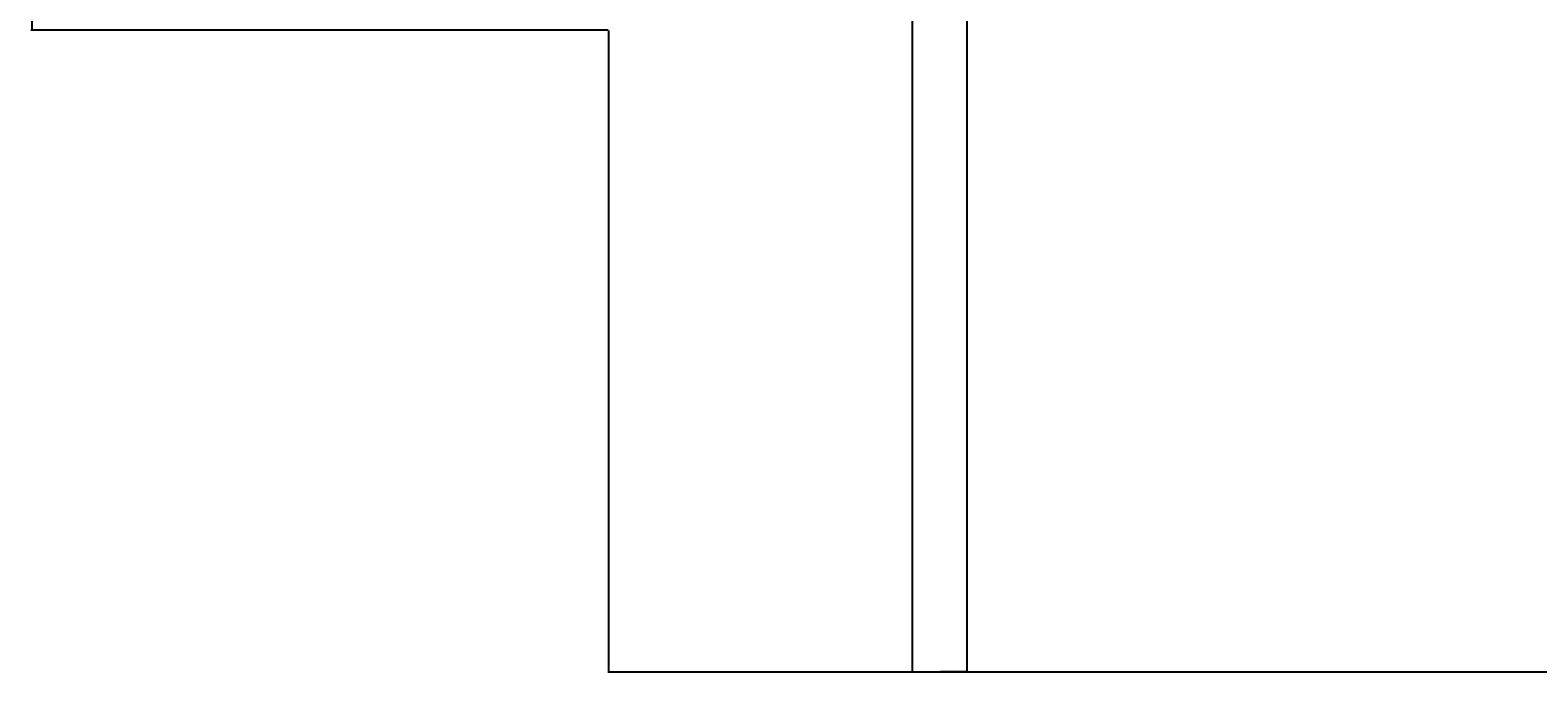
# Model space of a CAD drawing. Units: inches. Extents: x 5375 to 6084, y 16106 to 17259.
# Tile 1 of 32: x 5375 to 5624, y 16106 to 16212. Entities that reach past the tile are written whole.
import ezdxf

# ---------------------------------------------------------------- set-up
doc = ezdxf.new("R2010")
doc.units = ezdxf.units.IN
doc.layers.add('A-ANNO-DIMS', color=2, linetype='Continuous', lineweight=18)
doc.styles.get("Standard").update_dxf_attribs({"font": 'arial.ttf'})
doc.dimstyles.get("Standard").update_dxf_attribs({"dimtxt": 0.18, "dimasz": 0.18, "dimexe": 0.18, "dimexo": 0.0625, "dimgap": 0.09, "dimtad": 0, "dimtih": 1, "dimtoh": 1, "dimdec": 4, "dimzin": 0, "dimdsep": 46, "dimtxsty": 'Standard', "dimcen": 0.09, "dimadec": 0, "dimazin": 0, "dimtfac": 1, "dimtdec": 4, "dimtofl": 0, "dimtmove": 0, "dimatfit": 3, "dimfxl": 1, "dimtolj": 1, "dimtzin": 0, "dimarcsym": 0})

# ---------------------------------------------------------------- blocks, each defined once
blk = doc.blocks.new('*D30')
at = {"layer": 'A-ANNO-DIMS', "color": 0, "lineweight": -2, "transparency": 16777216}
for p, q in [((5470.62, 16212.32), (5470.62, 16106.48)), ((6031.62, 16212.32), (6031.62, 16106.48)), ((5470.8, 16106.66), (5750.85, 16106.66)), ((6031.44, 16106.66), (5751.39, 16106.66))]:
    blk.add_line(p, q, dxfattribs=at)
at = {"layer": 'A-ANNO-DIMS', "color": 0, "transparency": 16777216}
for points in [[(5470.8, 16106.69), (5470.8, 16106.63), (5470.62, 16106.66)], [(6031.44, 16106.69), (6031.44, 16106.63), (6031.62, 16106.66)]]:
    blk.add_solid(points, dxfattribs=at)
at = {"layer": 'Defpoints', "color": 0, "transparency": 16777216}
for p in [(5470.62, 16212.38), (6031.62, 16212.38), (6031.62, 16106.66)]:
    blk.add_point(p, dxfattribs=at)
at = {"layer": 'A-ANNO-DIMS', "color": 0, "transparency": 16777216, "insert": (5751.12, 16106.66), "char_height": 0.18, "attachment_point": 5}
blk.add_mtext('\\A1;561', dxfattribs=at)
blk = doc.blocks.new('*D33')
at = {"layer": 'A-ANNO-DIMS', "color": 0, "lineweight": -2, "transparency": 16777216}
for p, q in [((5470.56, 16360.58), (5375.56, 16360.58)), ((5375.74, 16360.4), (5375.74, 16286.66)), ((5375.74, 16212.56), (5375.74, 16286.3)), ((5470.56, 16212.38), (5375.56, 16212.38))]:
    blk.add_line(p, q, dxfattribs=at)
at = {"layer": 'A-ANNO-DIMS', "color": 0, "transparency": 16777216}
for points in [[(5375.71, 16360.4), (5375.77, 16360.4), (5375.74, 16360.58)], [(5375.71, 16212.56), (5375.77, 16212.56), (5375.74, 16212.38)]]:
    blk.add_solid(points, dxfattribs=at)
at = {"layer": 'Defpoints', "color": 0, "transparency": 16777216}
for p in [(5375.74, 16360.58), (5470.62, 16360.58), (5470.62, 16212.38)]:
    blk.add_point(p, dxfattribs=at)
at = {"layer": 'A-ANNO-DIMS', "color": 0, "transparency": 16777216, "insert": (5375.74, 16286.48), "char_height": 0.18, "attachment_point": 5}
blk.add_mtext('\\A1;148.2', dxfattribs=at)
blk = doc.blocks.new('*D40')
at = {"layer": 'A-ANNO-DIMS', "color": 0, "lineweight": -2, "transparency": 16777216}
for p, q in [((5529.62, 16876.52), (5529.62, 16106.48)), ((5520.62, 16867.52), (5520.62, 16106.48)), ((5520.8, 16106.66), (5524.97, 16106.66)), ((5529.44, 16106.66), (5525.27, 16106.66))]:
    blk.add_line(p, q, dxfattribs=at)
at = {"layer": 'A-ANNO-DIMS', "color": 0, "transparency": 16777216}
for points in [[(5520.8, 16106.69), (5520.8, 16106.63), (5520.62, 16106.66)], [(5529.44, 16106.69), (5529.44, 16106.63), (5529.62, 16106.66)]]:
    blk.add_solid(points, dxfattribs=at)
at = {"layer": 'Defpoints', "color": 0, "transparency": 16777216}
for p in [(5529.62, 16876.58), (5520.62, 16867.58), (5529.62, 16106.66)]:
    blk.add_point(p, dxfattribs=at)
at = {"layer": 'A-ANNO-DIMS', "color": 0, "transparency": 16777216, "insert": (5525.12, 16106.66), "char_height": 0.18, "attachment_point": 5}
blk.add_mtext('\\A1;9', dxfattribs=at)

msp = doc.modelspace()

# ---------------------------------------------------------------- dimensions: what is measured, and where the dimension line sits
at = {"layer": 'A-ANNO-DIMS'}
for base, p1, p2, picture, middle in [((5529.6199, 16106.6631), (5520.6199, 16867.5793), (5529.6199, 16876.5793), '*D40', (5525.1199, 16106.6631)), ((6031.6199, 16106.6631), (5470.6199, 16212.3785), (6031.6199, 16212.3785), '*D30', (5751.1199, 16106.6631))]:
    dim = msp.add_linear_dim(base=base, p1=p1, p2=p2, dimstyle='Standard', override={"dimdec": 0, "dimlfac": 1, "dimrnd": 0, "dimzin": 0, "dimdsep": 46, "dimlunit": 2}, dxfattribs=at)
    dim.commit()
    dim.dimension.update_dxf_attribs({"geometry": picture, "text_midpoint": middle})
dim = msp.add_linear_dim(base=(5375.7423, 16360.5793), p1=(5470.6199, 16212.3785), p2=(5470.6199, 16360.5793), angle=90, dimstyle='Standard', override={"dimdec": 1, "dimlfac": 1, "dimrnd": 0, "dimzin": 0, "dimdsep": 46, "dimlunit": 2}, dxfattribs=at)
dim.commit()
dim.dimension.update_dxf_attribs({"geometry": '*D33', "text_midpoint": (5375.7423, 16286.4789)})

doc.saveas('drawing.dxf')
